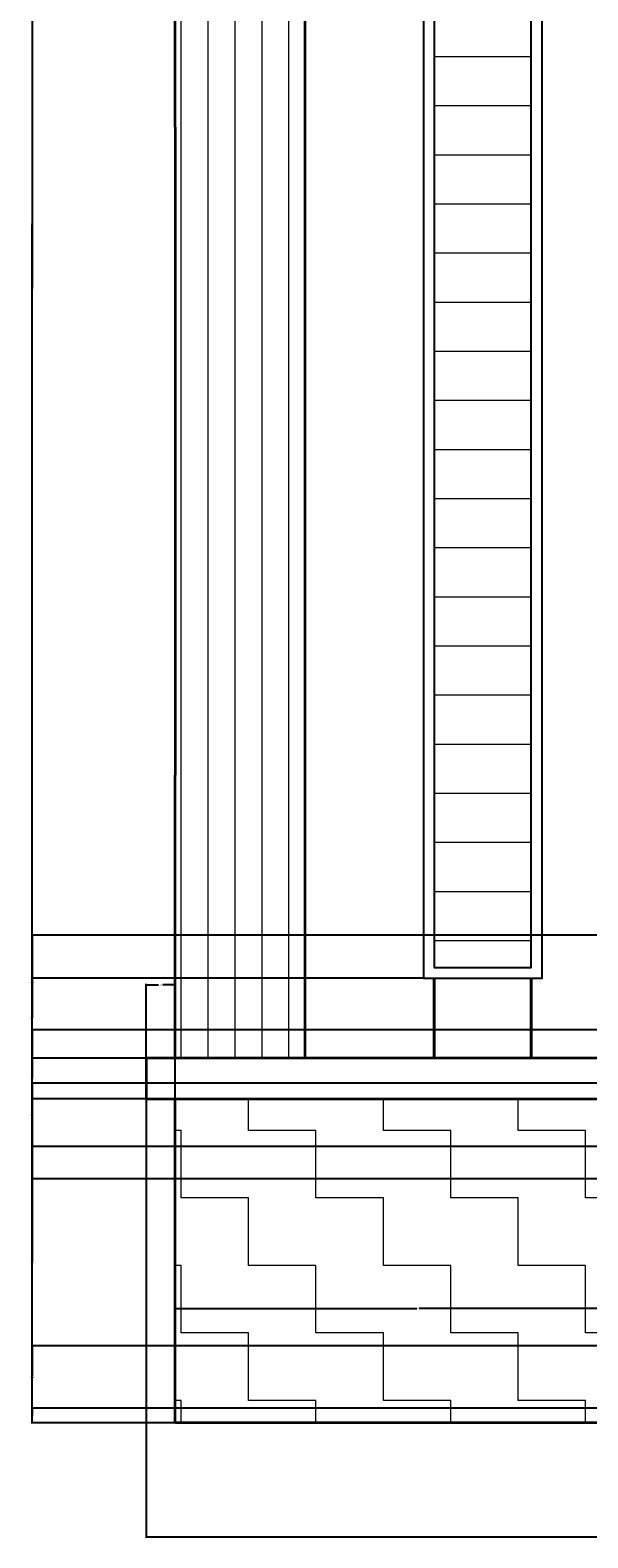
# Model space of a CAD drawing. Units: inches. Extents: x -3 to 302, y -138 to 325.
# Tile 1 of 5: x -3 to 100, y -138 to 141. Entities that reach past the tile are written whole.
import ezdxf

# ---------------------------------------------------------------- set-up
doc = ezdxf.new("R2010")
doc.units = ezdxf.units.IN
doc.header["$MEASUREMENT"] = 0
for name, color, linetype, lineweight in [('A-ANNO-DIMS', 2, 'Continuous', 18), ('A-ELEV', 7, 'Continuous', 35), ('A-ELEV-PATT', 8, 'Continuous', 13), ('A-GLAZ', 3, 'Continuous', 25)]:
    doc.layers.add(name, color=color, linetype=linetype, lineweight=lineweight)
doc.styles.get("Standard").update_dxf_attribs({"font": 'arial.ttf'})
doc.dimstyles.get("Standard").update_dxf_attribs({"dimtxt": 0.18, "dimasz": 0.18, "dimexe": 0.18, "dimexo": 0.0625, "dimgap": 0.09, "dimtad": 0, "dimtih": 1, "dimtoh": 1, "dimdec": 4, "dimzin": 0, "dimdsep": 46, "dimtxsty": 'Standard', "dimcen": 0.09, "dimadec": 0, "dimazin": 0, "dimtfac": 1, "dimtdec": 4, "dimtofl": 0, "dimtmove": 0, "dimatfit": 3, "dimfxl": 1, "dimtolj": 1, "dimtzin": 0, "dimarcsym": 0})

# ---------------------------------------------------------------- blocks, each defined once
blk = doc.blocks.new('*D17')
at = {"layer": 'A-ANNO-DIMS', "color": 0, "lineweight": -2, "transparency": 16777216}
for p, q in [((18.53, -56.69), (18.53, -137.96)), ((280.59, -116.69), (280.59, -137.96)), ((18.71, -137.78), (149.1, -137.78)), ((280.41, -137.78), (150.03, -137.78))]:
    blk.add_line(p, q, dxfattribs=at)
at = {"layer": 'A-ANNO-DIMS', "color": 0, "transparency": 16777216}
for points in [[(18.71, -137.75), (18.71, -137.81), (18.53, -137.78)], [(280.41, -137.75), (280.41, -137.81), (280.59, -137.78)]]:
    blk.add_solid(points, dxfattribs=at)
at = {"layer": 'Defpoints', "color": 0, "transparency": 16777216}
for p in [(18.53, -56.63), (280.59, -116.63), (280.59, -137.78)]:
    blk.add_point(p, dxfattribs=at)
at = {"layer": 'A-ANNO-DIMS', "color": 0, "transparency": 16777216, "insert": (149.56, -137.78), "char_height": 0.18, "attachment_point": 5}
blk.add_mtext('\\A1;262.06', dxfattribs=at)
blk = doc.blocks.new('*D18')
at = {"layer": 'A-ANNO-DIMS', "color": 0, "lineweight": -2, "transparency": 16777216}
for p, q in [((23.86, 303.37), (-2.8, 303.37)), ((-2.62, 303.19), (-2.62, 93.56)), ((-2.62, -116.45), (-2.62, 93.19)), ((23.86, -116.63), (-2.8, -116.63))]:
    blk.add_line(p, q, dxfattribs=at)
at = {"layer": 'A-ANNO-DIMS', "color": 0, "transparency": 16777216}
for points in [[(-2.65, 303.19), (-2.59, 303.19), (-2.62, 303.37)], [(-2.65, -116.45), (-2.59, -116.45), (-2.62, -116.63)]]:
    blk.add_solid(points, dxfattribs=at)
at = {"layer": 'Defpoints', "color": 0, "transparency": 16777216}
for p in [(-2.62, 303.37), (23.92, 303.37), (23.92, -116.63)]:
    blk.add_point(p, dxfattribs=at)
at = {"layer": 'A-ANNO-DIMS', "color": 0, "transparency": 16777216, "insert": (-2.62, 93.37), "char_height": 0.18, "attachment_point": 5}
blk.add_mtext('\\A1;420', dxfattribs=at)
blk = doc.blocks.new('*D31')
at = {"layer": 'A-ANNO-DIMS', "color": 0, "lineweight": -2, "transparency": 16777216}
for p, q in [((18.53, -56.56), (18.53, -35.3)), ((18.71, -35.48), (20.83, -35.48)), ((23.74, -35.48), (21.62, -35.48)), ((23.92, -56.56), (23.92, -35.3))]:
    blk.add_line(p, q, dxfattribs=at)
at = {"layer": 'A-ANNO-DIMS', "color": 0, "transparency": 16777216}
for points in [[(18.71, -35.45), (18.71, -35.51), (18.53, -35.48)], [(23.74, -35.45), (23.74, -35.51), (23.92, -35.48)]]:
    blk.add_solid(points, dxfattribs=at)
at = {"layer": 'Defpoints', "color": 0, "transparency": 16777216}
for p in [(23.92, -35.48), (18.53, -56.63), (23.92, -56.63)]:
    blk.add_point(p, dxfattribs=at)
at = {"layer": 'A-ANNO-DIMS', "color": 0, "transparency": 16777216, "insert": (21.23, -35.48), "char_height": 0.18, "attachment_point": 5}
blk.add_mtext('\\A1;5.392', dxfattribs=at)
blk = doc.blocks.new('*D32')
at = {"layer": 'A-ANNO-DIMS', "color": 0, "lineweight": -2, "transparency": 16777216}
for p, q in [((23.92, -116.56), (23.92, -95.3)), ((24.1, -95.48), (68.7, -95.48)), ((113.74, -95.48), (69.14, -95.48)), ((113.92, -116.56), (113.92, -95.3))]:
    blk.add_line(p, q, dxfattribs=at)
at = {"layer": 'A-ANNO-DIMS', "color": 0, "transparency": 16777216}
for points in [[(24.1, -95.45), (24.1, -95.51), (23.92, -95.48)], [(113.74, -95.45), (113.74, -95.51), (113.92, -95.48)]]:
    blk.add_solid(points, dxfattribs=at)
at = {"layer": 'Defpoints', "color": 0, "transparency": 16777216}
for p in [(113.92, -95.48), (23.92, -116.63), (113.92, -116.63)]:
    blk.add_point(p, dxfattribs=at)
at = {"layer": 'A-ANNO-DIMS', "color": 0, "transparency": 16777216, "insert": (68.92, -95.48), "char_height": 0.18, "attachment_point": 5}
blk.add_mtext('\\A1;90', dxfattribs=at)
blk = doc.blocks.new('*D34')
at = {"layer": 'A-ANNO-DIMS', "color": 0, "lineweight": -2, "transparency": 16777216}
for p, q in [((23.86, -56.63), (-2.8, -56.63)), ((-2.62, -56.81), (-2.62, -86.44)), ((-2.62, -116.45), (-2.62, -86.81)), ((23.86, -116.63), (-2.8, -116.63))]:
    blk.add_line(p, q, dxfattribs=at)
at = {"layer": 'A-ANNO-DIMS', "color": 0, "transparency": 16777216}
for points in [[(-2.65, -56.81), (-2.59, -56.81), (-2.62, -56.63)], [(-2.65, -116.45), (-2.59, -116.45), (-2.62, -116.63)]]:
    blk.add_solid(points, dxfattribs=at)
at = {"layer": 'Defpoints', "color": 0, "transparency": 16777216}
for p in [(-2.62, -56.63), (23.92, -56.63), (23.92, -116.63)]:
    blk.add_point(p, dxfattribs=at)
at = {"layer": 'A-ANNO-DIMS', "color": 0, "transparency": 16777216, "insert": (-2.62, -86.63), "char_height": 0.18, "attachment_point": 5}
blk.add_mtext('\\A1;60', dxfattribs=at)
blk = doc.blocks.new('*D35')
at = {"layer": 'A-ANNO-DIMS', "color": 0, "lineweight": -2, "transparency": 16777216}
for p, q in [((18.47, -49.09), (-2.8, -49.09)), ((-2.62, -49.27), (-2.62, -52.68)), ((-2.62, -56.45), (-2.62, -53.04)), ((18.47, -56.63), (-2.8, -56.63))]:
    blk.add_line(p, q, dxfattribs=at)
at = {"layer": 'A-ANNO-DIMS', "color": 0, "transparency": 16777216}
for points in [[(-2.65, -49.27), (-2.59, -49.27), (-2.62, -49.09)], [(-2.65, -56.45), (-2.59, -56.45), (-2.62, -56.63)]]:
    blk.add_solid(points, dxfattribs=at)
at = {"layer": 'Defpoints', "color": 0, "transparency": 16777216}
for p in [(-2.62, -49.09), (18.53, -49.09), (18.53, -56.63)]:
    blk.add_point(p, dxfattribs=at)
at = {"layer": 'A-ANNO-DIMS', "color": 0, "transparency": 16777216, "insert": (-2.62, -52.86), "char_height": 0.18, "attachment_point": 5}
blk.add_mtext('\\A1;7.533', dxfattribs=at)
blk = doc.blocks.new('*D36')
at = {"layer": 'A-ANNO-DIMS', "color": 0, "lineweight": -2, "transparency": 16777216}
for p, q in [((69.86, -34.27), (-2.8, -34.27)), ((-2.62, -34.45), (-2.62, -41.5)), ((-2.62, -48.91), (-2.62, -41.86)), ((71.86, -49.09), (-2.8, -49.09))]:
    blk.add_line(p, q, dxfattribs=at)
at = {"layer": 'A-ANNO-DIMS', "color": 0, "transparency": 16777216}
for points in [[(-2.65, -34.45), (-2.59, -34.45), (-2.62, -34.27)], [(-2.65, -48.91), (-2.59, -48.91), (-2.62, -49.09)]]:
    blk.add_solid(points, dxfattribs=at)
at = {"layer": 'Defpoints', "color": 0, "transparency": 16777216}
for p in [(-2.62, -34.27), (69.92, -34.27), (71.92, -49.09)]:
    blk.add_point(p, dxfattribs=at)
at = {"layer": 'A-ANNO-DIMS', "color": 0, "transparency": 16777216, "insert": (-2.62, -41.68), "char_height": 0.18, "attachment_point": 5}
blk.add_mtext('\\A1;14.82', dxfattribs=at)
blk = doc.blocks.new('*D37')
at = {"layer": 'A-ANNO-DIMS', "color": 0, "lineweight": -2, "transparency": 16777216}
for p, q in [((69.86, 245.37), (-2.8, 245.37)), ((-2.62, 245.19), (-2.62, 105.73)), ((-2.62, -34.09), (-2.62, 105.37)), ((69.86, -34.27), (-2.8, -34.27))]:
    blk.add_line(p, q, dxfattribs=at)
at = {"layer": 'A-ANNO-DIMS', "color": 0, "transparency": 16777216}
for points in [[(-2.65, 245.19), (-2.59, 245.19), (-2.62, 245.37)], [(-2.65, -34.09), (-2.59, -34.09), (-2.62, -34.27)]]:
    blk.add_solid(points, dxfattribs=at)
at = {"layer": 'Defpoints', "color": 0, "transparency": 16777216}
for p in [(-2.62, 245.37), (69.92, 245.37), (69.92, -34.27)]:
    blk.add_point(p, dxfattribs=at)
at = {"layer": 'A-ANNO-DIMS', "color": 0, "transparency": 16777216, "insert": (-2.62, 105.55), "char_height": 0.18, "attachment_point": 5}
blk.add_mtext('\\A1;279.65', dxfattribs=at)
blk = doc.blocks.new('*D76')
at = {"layer": 'A-ANNO-DIMS', "color": 0, "lineweight": -2, "transparency": 16777216}
for p, q in [((132.57, -113.96), (-2.8, -113.96)), ((-2.62, -114.14), (-2.62, -115.11)), ((130.43, -116.63), (-2.8, -116.63)), ((-2.62, -116.45), (-2.62, -115.48))]:
    blk.add_line(p, q, dxfattribs=at)
at = {"layer": 'A-ANNO-DIMS', "color": 0, "transparency": 16777216}
for points in [[(-2.65, -114.14), (-2.59, -114.14), (-2.62, -113.96)], [(-2.65, -116.45), (-2.59, -116.45), (-2.62, -116.63)]]:
    blk.add_solid(points, dxfattribs=at)
at = {"layer": 'Defpoints', "color": 0, "transparency": 16777216}
for p in [(-2.62, -113.96), (132.63, -113.96), (130.49, -116.63)]:
    blk.add_point(p, dxfattribs=at)
at = {"layer": 'A-ANNO-DIMS', "color": 0, "transparency": 16777216, "insert": (-2.62, -115.29), "char_height": 0.18, "attachment_point": 5}
blk.add_mtext('\\A1;2.661', dxfattribs=at)
blk = doc.blocks.new('*D77')
at = {"layer": 'A-ANNO-DIMS', "color": 0, "lineweight": -2, "transparency": 16777216}
for p, q in [((130.43, -102.38), (-2.8, -102.38)), ((-2.62, -102.56), (-2.62, -107.99)), ((-2.62, -113.78), (-2.62, -108.36)), ((132.57, -113.96), (-2.8, -113.96))]:
    blk.add_line(p, q, dxfattribs=at)
at = {"layer": 'A-ANNO-DIMS', "color": 0, "transparency": 16777216}
for points in [[(-2.65, -102.56), (-2.59, -102.56), (-2.62, -102.38)], [(-2.65, -113.78), (-2.59, -113.78), (-2.62, -113.96)]]:
    blk.add_solid(points, dxfattribs=at)
at = {"layer": 'Defpoints', "color": 0, "transparency": 16777216}
for p in [(-2.62, -102.38), (130.49, -102.38), (132.63, -113.96)]:
    blk.add_point(p, dxfattribs=at)
at = {"layer": 'A-ANNO-DIMS', "color": 0, "transparency": 16777216, "insert": (-2.62, -108.17), "char_height": 0.18, "attachment_point": 5}
blk.add_mtext('\\A1;11.582', dxfattribs=at)
blk = doc.blocks.new('*D78')
at = {"layer": 'A-ANNO-DIMS', "color": 0, "lineweight": -2, "transparency": 16777216}
for p, q in [((130.43, -71.46), (-2.8, -71.46)), ((-2.62, -71.64), (-2.62, -86.74)), ((-2.62, -102.2), (-2.62, -87.1)), ((130.43, -102.38), (-2.8, -102.38))]:
    blk.add_line(p, q, dxfattribs=at)
at = {"layer": 'A-ANNO-DIMS', "color": 0, "transparency": 16777216}
for points in [[(-2.65, -71.64), (-2.59, -71.64), (-2.62, -71.46)], [(-2.65, -102.2), (-2.59, -102.2), (-2.62, -102.38)]]:
    blk.add_solid(points, dxfattribs=at)
at = {"layer": 'Defpoints', "color": 0, "transparency": 16777216}
for p in [(-2.62, -71.46), (130.49, -71.46), (130.49, -102.38)]:
    blk.add_point(p, dxfattribs=at)
at = {"layer": 'A-ANNO-DIMS', "color": 0, "transparency": 16777216, "insert": (-2.62, -86.92), "char_height": 0.18, "attachment_point": 5}
blk.add_mtext('\\A1;30.926', dxfattribs=at)
blk = doc.blocks.new('*D79')
at = {"layer": 'A-ANNO-DIMS', "color": 0, "lineweight": -2, "transparency": 16777216}
for p, q in [((132.57, -53.73), (-2.8, -53.73)), ((-2.62, -53.91), (-2.62, -59.4)), ((-2.62, -65.25), (-2.62, -59.76)), ((130.43, -65.43), (-2.8, -65.43))]:
    blk.add_line(p, q, dxfattribs=at)
at = {"layer": 'A-ANNO-DIMS', "color": 0, "transparency": 16777216}
for points in [[(-2.65, -53.91), (-2.59, -53.91), (-2.62, -53.73)], [(-2.65, -65.25), (-2.59, -65.25), (-2.62, -65.43)]]:
    blk.add_solid(points, dxfattribs=at)
at = {"layer": 'Defpoints', "color": 0, "transparency": 16777216}
for p in [(-2.62, -53.73), (132.63, -53.73), (130.49, -65.43)]:
    blk.add_point(p, dxfattribs=at)
at = {"layer": 'A-ANNO-DIMS', "color": 0, "transparency": 16777216, "insert": (-2.62, -59.58), "char_height": 0.18, "attachment_point": 5}
blk.add_mtext('\\A1;11.695', dxfattribs=at)
blk = doc.blocks.new('*D80')
at = {"layer": 'A-ANNO-DIMS', "color": 0, "lineweight": -2, "transparency": 16777216}
for p, q in [((130.43, -43.86), (-2.8, -43.86)), ((-2.62, -44.04), (-2.62, -48.61)), ((-2.62, -53.55), (-2.62, -48.98)), ((132.57, -53.73), (-2.8, -53.73))]:
    blk.add_line(p, q, dxfattribs=at)
at = {"layer": 'A-ANNO-DIMS', "color": 0, "transparency": 16777216}
for points in [[(-2.65, -44.04), (-2.59, -44.04), (-2.62, -43.86)], [(-2.65, -53.55), (-2.59, -53.55), (-2.62, -53.73)]]:
    blk.add_solid(points, dxfattribs=at)
at = {"layer": 'Defpoints', "color": 0, "transparency": 16777216}
for p in [(-2.62, -43.86), (130.49, -43.86), (132.63, -53.73)]:
    blk.add_point(p, dxfattribs=at)
at = {"layer": 'A-ANNO-DIMS', "color": 0, "transparency": 16777216, "insert": (-2.62, -48.79), "char_height": 0.18, "attachment_point": 5}
blk.add_mtext('\\A1;9.876', dxfattribs=at)
blk = doc.blocks.new('*D81')
at = {"layer": 'A-ANNO-DIMS', "color": 0, "lineweight": -2, "transparency": 16777216}
for p, q in [((131.72, -26.3), (-2.8, -26.3)), ((-2.62, -26.48), (-2.62, -34.9)), ((-2.62, -43.68), (-2.62, -35.26)), ((130.43, -43.86), (-2.8, -43.86))]:
    blk.add_line(p, q, dxfattribs=at)
at = {"layer": 'A-ANNO-DIMS', "color": 0, "transparency": 16777216}
for points in [[(-2.65, -26.48), (-2.59, -26.48), (-2.62, -26.3)], [(-2.65, -43.68), (-2.59, -43.68), (-2.62, -43.86)]]:
    blk.add_solid(points, dxfattribs=at)
at = {"layer": 'Defpoints', "color": 0, "transparency": 16777216}
for p in [(-2.62, -26.3), (131.79, -26.3), (130.49, -43.86)]:
    blk.add_point(p, dxfattribs=at)
at = {"layer": 'A-ANNO-DIMS', "color": 0, "transparency": 16777216, "insert": (-2.62, -35.08), "char_height": 0.18, "attachment_point": 5}
blk.add_mtext('\\A1;17.553', dxfattribs=at)

msp = doc.modelspace()

# ---------------------------------------------------------------- hatches: boundary and pattern name
at = {"layer": 'A-ELEV-PATT'}
h = msp.add_hatch(dxfattribs=at)
h.set_pattern_fill('_USER', color=256, scale=5, angle=90, pattern_type=0)
h.set_pattern_definition([(90, (0, 0), (-5, 3e-16), [])])
h.paths.add_polyline_path([(47.922, 303.3747), (23.922, 303.3747), (23.922, 123.3747), (23.922, 3.3747), (23.922, -49.0923), (47.922, -49.0923)])
h = msp.add_hatch(dxfattribs=at)
h.set_pattern_fill('_USER', color=256, scale=9.1, pattern_type=0)
h.set_pattern_definition([(0, (0, 0), (0, 9.1), [])])
h.paths.add_polyline_path([(89.922, 243.3747), (71.922, 243.3747), (71.922, -32.2717), (89.922, -32.2717)])
h = msp.add_hatch(dxfattribs=at)
h.set_pattern_fill('ZIGZAG', color=256, scale=100, angle=90)
h.set_pattern_definition([(90, (0, 0), (-12.5, 12.5), [12.5, -12.5]), (180, (8e-16, 12.5), (-12.5, -12.5), [12.5, -12.5])])
h.paths.add_polyline_path([(113.922, -56.6253), (23.922, -56.6253), (23.922, -116.6253), (113.922, -116.6253)])

# ---------------------------------------------------------------- linework, layer by layer
at = {"layer": 'A-ELEV'}
for p, q in [((23.922, 123.3747), (23.922, 303.3747)), ((47.922, 303.3747), (47.922, -49.0923)), ((23.922, 123.3747), (23.922, 3.3747)), ((23.922, -49.0923), (23.922, 3.3747)), ((71.922, -49.0923), (71.922, -34.2717)), ((71.922, -34.2717), (71.922, -49.0923)), ((89.922, -49.0923), (89.922, -34.2717)), ((89.922, -34.2717), (89.922, -49.0923)), ((89.922, -49.0923), (71.922, -49.0923)), ((23.922, -116.6253), (23.922, -56.6253)), ((23.922, -56.6253), (113.922, -56.6253)), ((263.922, -116.6253), (23.922, -116.6253))]:
    msp.add_line(p, q, dxfattribs=at)
msp.add_lwpolyline([(113.922, -49.0923), (18.5303, -49.0923), (18.5303, -56.6253), (113.922, -56.6253)], dxfattribs=at)
at = {"layer": 'A-GLAZ'}
for points in [[(69.922, 245.3747), (69.922, -34.2717), (91.922, -34.2717), (91.922, 245.3747)], [(71.922, 243.3747), (71.922, -32.2717), (89.922, -32.2717), (89.922, 243.3747)]]:
    msp.add_lwpolyline(points, close=True, dxfattribs=at)

# ---------------------------------------------------------------- dimensions: what is measured, and where the dimension line sits
at = {"layer": 'A-ANNO-DIMS'}
for base, p1, p2, override, picture, middle in [((-2.6197, 303.3747), (23.922, -116.6253), (23.922, 303.3747), {"dimdec": 0, "dimlfac": 1, "dimrnd": 0, "dimzin": 0, "dimdsep": 46, "dimlunit": 2}, '*D18', (-2.6197, 93.3747)), ((-2.6197, 245.3747), (69.922, -34.2717), (69.922, 245.3747), {"dimdec": 2, "dimlfac": 1, "dimrnd": 0, "dimzin": 0, "dimdsep": 46, "dimlunit": 2}, '*D37', (-2.6197, 105.5515)), ((-2.61974, -26.30337), (130.48946, -43.85589), (131.7871, -26.30337), {"dimdec": 3, "dimlfac": 1, "dimrnd": 0, "dimzin": 0, "dimdsep": 46, "dimlunit": 2}, '*D81', (-2.61974, -35.07963)), ((-2.6197, -34.2717), (71.922, -49.0923), (69.922, -34.2717), {"dimdec": 2, "dimlfac": 1, "dimrnd": 0, "dimzin": 0, "dimdsep": 46, "dimlunit": 2}, '*D36', (-2.6197, -41.682)), ((-2.6197, -43.8559), (132.6328, -53.7317), (130.4895, -43.8559), {"dimdec": 3, "dimlfac": 1, "dimrnd": 0, "dimzin": 0, "dimdsep": 46, "dimlunit": 2}, '*D80', (-2.6197, -48.7938)), ((-2.6197, -49.0923), (18.5303, -56.6253), (18.5303, -49.0923), {"dimdec": 3, "dimlfac": 1, "dimrnd": 0, "dimzin": 0, "dimdsep": 46, "dimlunit": 2}, '*D35', (-2.6197, -52.8588)), ((-2.6197, -53.7317), (130.4895, -65.4264), (132.6328, -53.7317), {"dimdec": 3, "dimlfac": 1, "dimrnd": 0, "dimzin": 0, "dimdsep": 46, "dimlunit": 2}, '*D79', (-2.6197, -59.579)), ((-2.6197, -56.6253), (23.922, -116.6253), (23.922, -56.6253), {"dimdec": 0, "dimlfac": 1, "dimrnd": 0, "dimzin": 0, "dimdsep": 46, "dimlunit": 2}, '*D34', (-2.6197, -86.6253)), ((-2.6197, -71.4563), (130.4895, -102.3827), (130.4895, -71.4563), {"dimdec": 3, "dimlfac": 1, "dimrnd": 0, "dimzin": 0, "dimdsep": 46, "dimlunit": 2}, '*D78', (-2.6197, -86.9195)), ((-2.6197, -102.3827), (132.6328, -113.9645), (130.4895, -102.3827), {"dimdec": 3, "dimlfac": 1, "dimrnd": 0, "dimzin": 0, "dimdsep": 46, "dimlunit": 2}, '*D77', (-2.6197, -108.1736)), ((-2.6197, -113.9645), (130.4895, -116.6253), (132.6328, -113.9645), {"dimdec": 3, "dimlfac": 1, "dimrnd": 0, "dimzin": 0, "dimdsep": 46, "dimlunit": 2}, '*D76', (-2.6197, -115.2949))]:
    dim = msp.add_linear_dim(base=base, p1=p1, p2=p2, angle=90, dimstyle='Standard', override=override, dxfattribs=at)
    dim.commit()
    dim.dimension.update_dxf_attribs({"geometry": picture, "text_midpoint": middle})
for base, p1, p2, override, picture, middle in [((23.922, -35.4753), (18.5303, -56.6253), (23.922, -56.6253), {"dimdec": 3, "dimlfac": 1, "dimrnd": 0, "dimzin": 0, "dimdsep": 46, "dimlunit": 2}, '*D31', (21.2261, -35.4753)), ((280.5936, -137.7753), (18.5303, -56.6253), (280.5936, -116.6253), {"dimdec": 2, "dimlfac": 1, "dimrnd": 0, "dimzin": 0, "dimdsep": 46, "dimlunit": 2}, '*D17', (149.5619, -137.7753)), ((113.922, -95.4753), (23.922, -116.6253), (113.922, -116.6253), {"dimdec": 0, "dimlfac": 1, "dimrnd": 0, "dimzin": 0, "dimdsep": 46, "dimlunit": 2}, '*D32', (68.922, -95.4753))]:
    dim = msp.add_linear_dim(base=base, p1=p1, p2=p2, dimstyle='Standard', override=override, dxfattribs=at)
    dim.commit()
    dim.dimension.update_dxf_attribs({"geometry": picture, "text_midpoint": middle})

doc.saveas('drawing.dxf')
